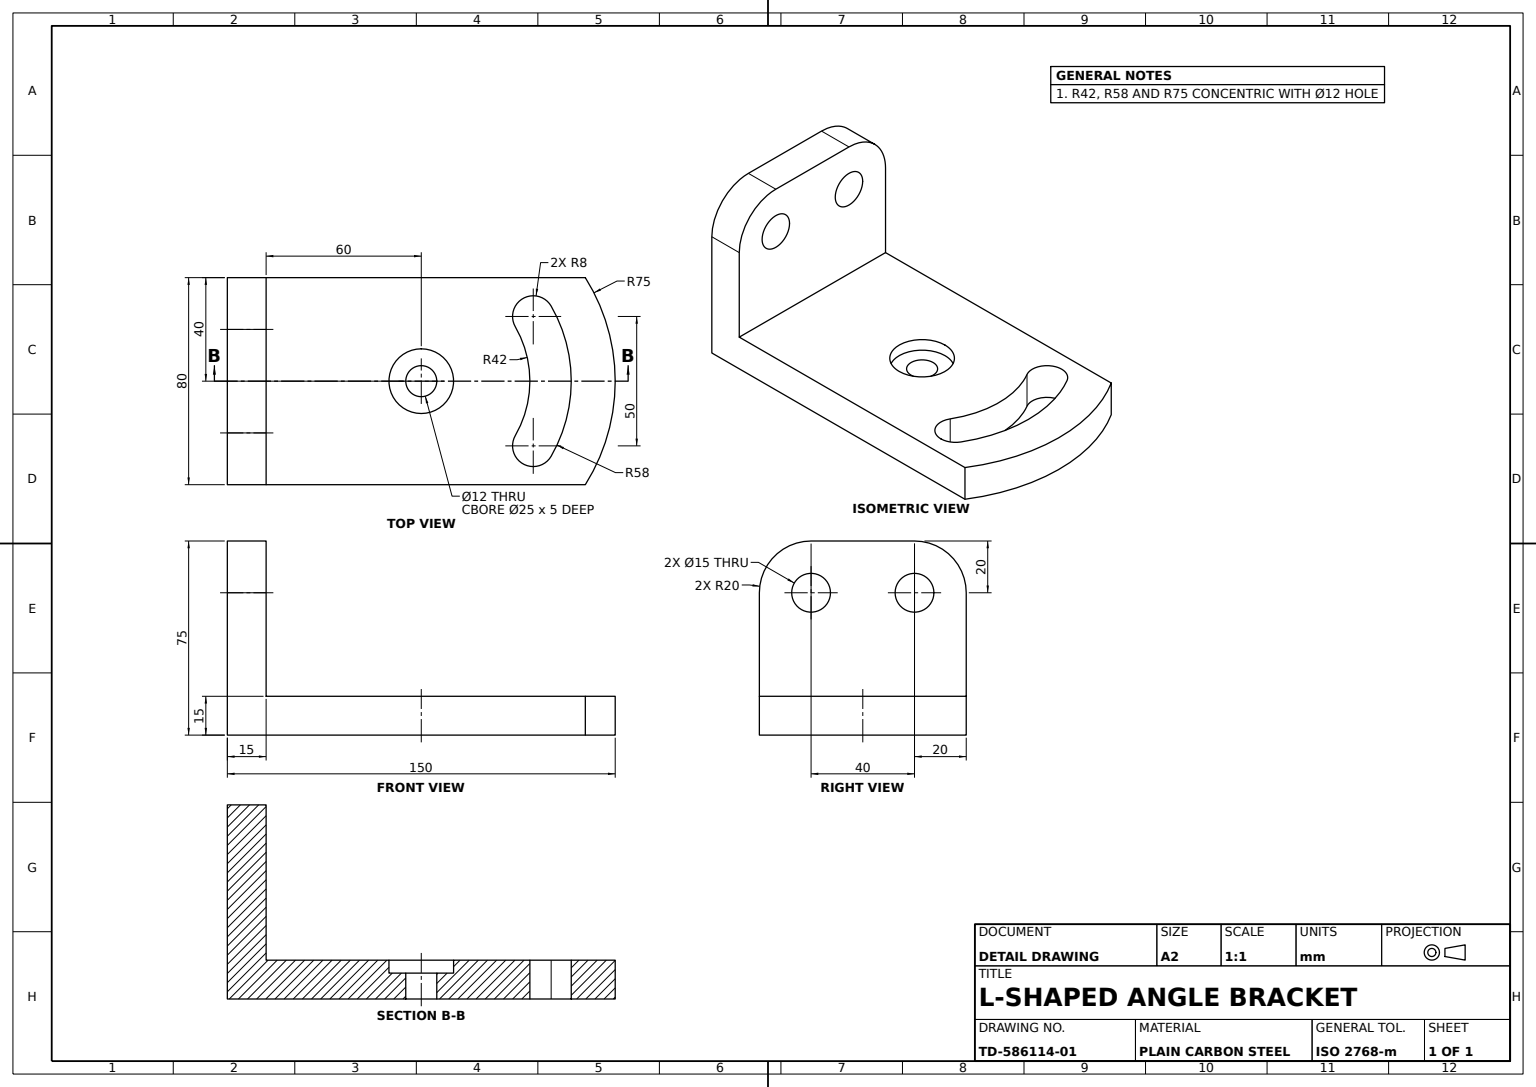
from build123d import *

# Parameters (mm, degrees)
BASE_PLATE_SKETCH_W             = 150
BASE_PLATE_SKETCH_H             = 80
BASE_PLATE_DEPTH                = 15
PROFILE_TRIM_CUT_DEPTH          = 35
COUNTERBORE_SKETCH_R            = 12.5
COUNTERBORE_SKETCH_R_2          = 6
COUNTERBORE_25X5_DEPTH          = 5
THROUGH_HOLE_SKETCH_R           = 6
THROUGH_HOLE_CUT_DEPTH          = 25
ARC_SLOT_8_R50_30DEG_DEPTH      = 86.586213843
ARC_SLOT_8_R50_30DEG_DEPTH_BACK = 86.586213843
UPRIGHT_FLANGE_SKETCH_R         = 7.5
UPRIGHT_FLANGE_DEPTH            = 15


with BuildPart() as part:
    # Base Plate Sketch → Base Plate (new body)
    with BuildSketch(Plane(origin=(0, 0, 0), x_dir=(1, 0, 0), z_dir=(0, 1, 0))):
        Rectangle(BASE_PLATE_SKETCH_W, BASE_PLATE_SKETCH_H)
    extrude(amount=BASE_PLATE_DEPTH)

    # Profile Trim Sketch → Profile Trim Cut (cut)
    with BuildSketch(Plane(origin=(0, 15, 0), x_dir=(1, 0, 0), z_dir=(0, 1, 0))):
        with BuildLine():
            Line((75, 0), (75, 40))
            Line((75, 40), (63.442887702, 40))
            ThreePointArc((63.442887702, 40), (72.052815967, 20.818062138), (75, 0))
        make_face()
        with BuildLine():
            Line((75, -40), (75, 0))
            ThreePointArc((75, 0), (72.052815967, -20.818062138), (63.442887702, -40))
            Line((63.442887702, -40), (75, -40))
        make_face()
    extrude(amount=-PROFILE_TRIM_CUT_DEPTH, mode=Mode.SUBTRACT)

    # Counterbore Sketch → Counterbore Ø25x5 (cut)
    with BuildSketch(Plane(origin=(0, 15, 0), x_dir=(1, 0, 0), z_dir=(0, 1, 0))):
        with Locations(Location((0, 0, 0), (0, 0, 270))):
            Circle(COUNTERBORE_SKETCH_R)
        with Locations(Location((0, 0, 0), (0, 0, 270))):
            Circle(COUNTERBORE_SKETCH_R_2, mode=Mode.SUBTRACT)
    extrude(amount=-COUNTERBORE_25X5_DEPTH, mode=Mode.SUBTRACT)

    # Through Hole Sketch → Through Hole Cut (cut)
    with BuildSketch(Plane(origin=(0, 15, 0), x_dir=(1, 0, 0), z_dir=(0, 1, 0))):
        with Locations(Location((0, 0, 0), (0, 0, 270))):
            Circle(THROUGH_HOLE_SKETCH_R)
    extrude(amount=-THROUGH_HOLE_CUT_DEPTH, mode=Mode.SUBTRACT)

    # Arc Slot Sketch → Arc Slot 8 R50 30deg (cut, two sides: drawn at the far end of the back side and taken through both)
    with BuildSketch(Plane(origin=(0, 10, 0), x_dir=(1, 0, 0), z_dir=(0, 1, 0)).offset(-ARC_SLOT_8_R50_30DEG_DEPTH_BACK)):
        with BuildLine():
            ThreePointArc((50.229473419, -29), (58, 0), (50.229473419, 29))
            ThreePointArc((50.229473419, 29), (39.301270189, 31.92820323), (36.373066959, 21))
            ThreePointArc((36.373066959, 21), (42, 0), (36.373066959, -21))
            ThreePointArc((36.373066959, -21), (39.301270189, -31.92820323), (50.229473419, -29))
        make_face()
    extrude(amount=ARC_SLOT_8_R50_30DEG_DEPTH + ARC_SLOT_8_R50_30DEG_DEPTH_BACK, mode=Mode.SUBTRACT)

    # Upright Flange Sketch → Upright Flange (add)
    with BuildSketch(Plane.ZY.offset(75)):
        with BuildLine():
            Line((-40, 15), (-40, 55))
            ThreePointArc((-40, 55), (-34.142135624, 69.142135624), (-20, 75))
            Line((-20, 75), (20, 75))
            ThreePointArc((20, 75), (34.142135624, 69.142135624), (40, 55))
            Line((40, 55), (40, 15))
            Line((40, 15), (-40, 15))
        make_face()
        with Locations((-20, 55)):
            Circle(UPRIGHT_FLANGE_SKETCH_R, mode=Mode.SUBTRACT)
        with Locations((20, 55)):
            Circle(UPRIGHT_FLANGE_SKETCH_R, mode=Mode.SUBTRACT)
    extrude(amount=-UPRIGHT_FLANGE_DEPTH)


solid = part.part
